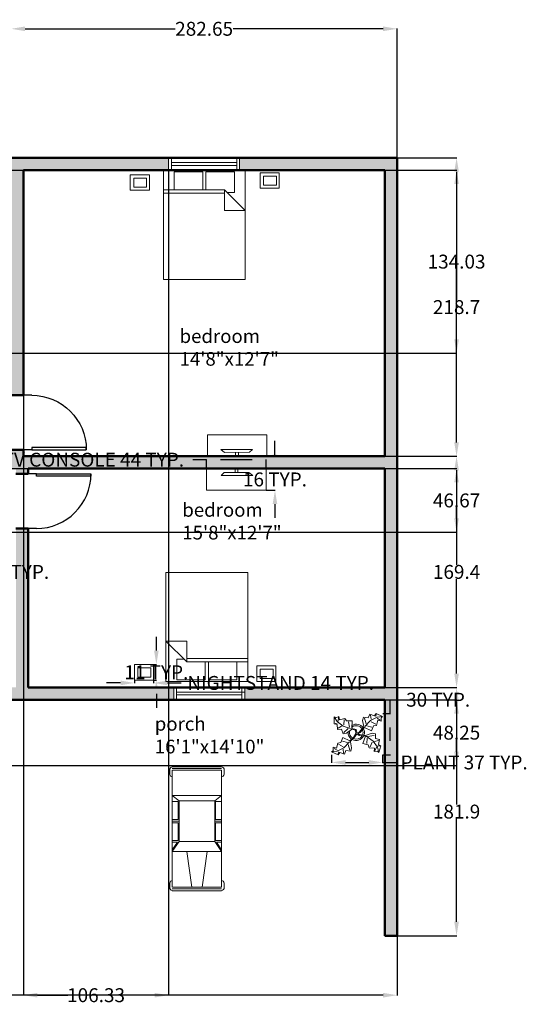
# Model space of a CAD drawing. Units: inches. Extents: x 12496 to 13538, y 6171 to 6892.
# Tile 6 of 6: x 13167 to 13538, y 6171 to 6892. Entities that reach past the tile are written whole.
import ezdxf

# ---------------------------------------------------------------- set-up
doc = ezdxf.new("R2010")
doc.units = ezdxf.units.IN
doc.header["$MEASUREMENT"] = 0
for name, color, linetype, lineweight in [('A-ANNO-DIMS', 2, 'Continuous', 18), ('A-AREA-IDEN', 7, 'Continuous', 25), ('A-DOOR', 3, 'Continuous', 25), ('A-EQPM-VEHI', 9, 'Continuous', 18), ('A-FURN', 8, 'Continuous', 18), ('A-GLAZ', 4, 'Continuous', 18), ('A-WALL', 7, 'Continuous', 50), ('L-PLNT', 3, 'Continuous', 18)]:
    doc.layers.add(name, color=color, linetype=linetype, lineweight=lineweight)
doc.layers.add('A-WALL-PATT', color=18, linetype='Continuous', lineweight=13, true_color=0x000000)
doc.styles.get("Standard").update_dxf_attribs({"font": 'arial.ttf'})
doc.dimstyles.get("Standard").update_dxf_attribs({"dimtxt": 10.18, "dimasz": 10.18, "dimexe": 0.18, "dimexo": 0.0625, "dimgap": 0.09, "dimtad": 0, "dimtih": 1, "dimtoh": 1, "dimdec": 0, "dimzin": 0, "dimdsep": 46, "dimlunit": 3, "dimtxsty": 'Standard', "dimcen": 0.09, "dimadec": 0, "dimazin": 0, "dimtfac": 1, "dimtdec": 0, "dimtofl": 0, "dimtmove": 0, "dimatfit": 3, "dimfxl": 1, "dimtolj": 1, "dimtzin": 0, "dimarcsym": 0})

# ---------------------------------------------------------------- blocks, each defined once
blk = doc.blocks.new('Bed - Queen')
for p, q in [((0, -80.00003), (0, 0)), ((0, 0), (59.99999, 0)), ((59.99999, 0), (59.99999, -80.00003)), ((7.99999, -1.2), (28.79998, -1.2)), ((7.99999, -14.4), (7.99999, -1.2)), ((28.79998, -1.2), (28.79998, -14.4)), ((31.19999, -1.2), (51.99999, -1.2)), ((31.19999, -14.4), (31.19999, -1.2)), ((51.99999, -1.2), (51.99999, -16.4)), ((0, -14.4), (44.8, -14.4)), ((59.99999, -29.6), (44.8, -14.4)), ((44.8, -14.4), (44.8, -29.6)), ((44.8, -16.8), (0, -16.8)), ((51.99999, -16.4), (46.79936, -16.4)), ((44.8, -29.6), (59.99999, -29.6)), ((59.99999, -80.00003), (0, -80.00003))]:
    blk.add_line(p, q)
blk = doc.blocks.new('Plant - Rubber or Philodendron')
for p, q in [((-16.2005, 11.4774), (-13.9899, 8.1064)), ((-16.2005, 11.4774), (-14.8639, 10.7964)), ((-16.0159, 6.3329), (-16.2005, 11.4774)), ((-14.8639, 10.7964), (-12.6195, 11.8975)), ((-13.9899, 8.1064), (-9.5434, 4.7185)), ((-13.3174, 8.325), (-13.0735, 11.0065)), ((-12.6195, 11.8975), (-12.1909, 9.4345)), ((-12.1909, 9.4345), (-8.3829, 10.3)), ((-8.8369, 9.409), (-9.0894, 5.6095)), ((-8.3829, 10.3), (-7.0549, 8.501)), ((-7.0549, 8.501), (-3.0284, 8.6941)), ((-4.8529, 4.012), (-5.7184, 7.82)), ((-3.0284, 8.6941), (-3.0709, 3.1041)), ((4.6914, 8.8812), (5.3859, 11.2828)), ((4.6914, 8.8812), (5.5014, 4.4831)), ((5.3859, 11.2828), (8.8871, 10.7908)), ((5.9878, 10.4842), (7.1971, 6.3869)), ((10.3916, 8.7942), (6.2847, 4.4028)), ((8.8871, 10.7908), (9.9809, 13.4933)), ((9.9809, 13.4933), (13.3837, 12.301)), ((15.3859, 11.3055), (10.3916, 8.7942)), ((10.5828, 12.6946), (10.8893, 9.7953)), ((14.2977, 6.1031), (10.9934, 7.9956)), ((13.3837, 12.301), (14.68, 13.9039)), ((14.5816, 13.2037), (14.3848, 11.8033)), ((14.68, 13.9039), (19.3848, 11.8146)), ((15.7909, 9.1065), (14.8995, 5.3044)), ((15.2875, 10.6053), (17.5907, 9.2105)), ((19.3848, 11.8146), (15.3859, 11.3055)), ((18.1925, 8.4119), (15.7909, 9.1065)), ((19.3848, 11.8146), (18.1868, 10.9119)), ((18.1868, 10.9119), (18.1925, 8.4119)), ((-14.0069, 5.8704), (-16.0159, 6.3329)), ((-15.3434, 6.5514), (-13.9984, 6.9884)), ((-13.5868, 2.2894), (-14.0069, 5.8704)), ((-10.6784, 2.491), (-13.5868, 2.2894)), ((-13.1329, 3.1804), (-10.6614, 4.727)), ((-9.5858, -0.8715), (-10.6784, 2.491)), ((-9.5434, 4.7185), (-4.1917, 2.9888)), ((-9.1318, 0.0195), (-5.9793, 2.9025)), ((-7.1228, -0.443), (-3.5248, 2.2131)), ((-3.5248, 2.2131), (-3.3011, 2.4355)), ((-3.3011, 2.4355), (-0.5306, 1.7947)), ((-3.0709, 3.1041), (0.0797, 2.3163)), ((-0.5306, 1.7947), (-0.2255, -0.5527)), ((-0.5306, 1.7947), (-0.5306, 1.7947)), ((0.0797, 2.3163), (0.4866, -0.031)), ((0.4866, -0.031), (2.1141, 0.2298)), ((2.1141, 0.2298), (5.4346, 3.9146)), ((6.1032, 3.6844), (2.8262, -0.031)), ((5.4346, 3.9146), (5.5014, 4.4831)), ((11.1089, 1.1958), (6.1032, 3.6844)), ((7.7005, 4.8881), (11.5025, 3.9967)), ((12.7005, 4.8994), (11.1089, 1.1958)), ((14.8995, 5.3044), (12.7005, 4.8994)), ((-11.3237, -7.2629), (-9.7321, -3.5593)), ((-6.3237, -7.2516), (-10.1257, -6.3602)), ((-9.7321, -3.5593), (-4.7264, -6.0479)), ((-7.1228, -0.443), (-9.5858, -0.8715)), ((-9.0148, -11.1577), (-4.9047, -6.8122)), ((-2.019, -3.6148), (-4.7264, -6.0479)), ((-4.1246, -6.8466), (-4.0579, -6.2781)), ((-3.3146, -11.2447), (-4.1246, -6.8466)), ((-4.0579, -6.2781), (-0.9375, -3.1608)), ((-2.019, -3.6148), (-0.2255, -0.5527)), ((-0.9375, -3.1608), (0.5883, -0.8135)), ((0.5883, -0.8135), (2.2447, -2.0916)), ((2.8262, -0.031), (1.3003, -0.5527)), ((1.3003, -0.5527), (2.4193, -1.4655)), ((2.2447, -2.0916), (6.7108, -2.6626)), ((2.4193, -1.4655), (6.895, -2.1175)), ((4.943, -7.9659), (6.7108, -2.6626)), ((11.6605, -0.5413), (6.895, -2.1175)), ((12.3677, -6.1981), (7.219, -2.6772)), ((8.125, -4.0768), (7.7715, -7.9659)), ((8.3544, -2.7453), (13.1973, -2.1704)), ((10.2463, -10.4408), (11.6605, -6.9053)), ((11.6605, -0.5413), (14.1354, -0.8948)), ((15.5496, -10.7943), (12.3677, -6.1981)), ((16.2567, -5.8446), (13.4283, -6.5517)), ((14.1354, -0.8948), (14.1354, -4.4304)), ((14.1354, -4.4304), (16.9638, -5.1375)), ((16.9638, -5.1375), (16.2567, -8.673)), ((-18.008, -14.1781), (-16.8101, -13.2754)), ((-18.008, -14.1781), (-14.0091, -13.669)), ((-13.3032, -16.2674), (-18.008, -14.1781)), ((-16.8157, -10.7754), (-14.4141, -11.4699)), ((-16.8101, -13.2754), (-16.8157, -10.7754)), ((-13.9107, -12.9688), (-16.2139, -11.574)), ((-14.4141, -11.4699), (-13.5228, -7.6679)), ((-14.0091, -13.669), (-9.0148, -11.1577)), ((-13.5228, -7.6679), (-11.3237, -7.2629)), ((-13.2048, -15.5672), (-13.008, -14.1668)), ((-12.921, -8.4665), (-9.6166, -10.359)), ((-9.206, -15.0581), (-9.5126, -12.1588)), ((-7.5103, -13.1543), (-8.6042, -15.8568)), ((-4.0092, -13.6463), (-7.5103, -13.1543)), ((-4.611, -12.8477), (-5.8203, -8.7504)), ((-3.3146, -11.2447), (-4.0092, -13.6463)), ((8.8321, -9.0266), (4.943, -7.9659)), ((9.5392, -11.1479), (8.8321, -9.0266)), ((13.4283, -11.5015), (9.5392, -11.1479)), ((13.0748, -13.9763), (13.4283, -11.5015)), ((15.5496, -13.6228), (13.0748, -13.9763)), ((14.8425, -10.7943), (13.7819, -13.2692)), ((16.6103, -14.6834), (15.5496, -10.7943)), ((16.6103, -14.6834), (15.5496, -13.6228)), ((17.3174, -9.7337), (15.9032, -9.7337)), ((16.2567, -8.673), (18.0245, -9.7337)), ((18.0245, -9.7337), (16.6103, -14.6834)), ((-12.0069, -14.6645), (-13.3032, -16.2674)), ((-8.6042, -15.8568), (-12.0069, -14.6645))]:
    blk.add_line(p, q)
for centre, radius, start, end in [((0.0308, 0.1664), 6, 178.6147, 235.1169), ((0.0308, 0.1664), 5, 168.1647, 238.6725), ((0, 0), 6.1275, 34.37569, 120.1028), ((-0.0601, -0.2075), 5.2461, 33.82192, 124.9414), ((-0.2664, 0.1682), 5.2775, 338.4094, 20.03007), ((-0.098, 0.1364), 6.1288, 341.2017, 26.09184), ((-0.0234, 0.3825), 6.1492, 242.5812, 331.2714), ((-0.1102, 0.4886), 5.2883, 247.3711, 327.472)]:
    blk.add_arc(centre, radius, start, end)
blk = doc.blocks.new('*U18')
for p, q in [((0.1, -0.4), (0.1, 38.3)), ((2.8, -0.4), (2.8, 38.3)), ((5.4, 42.3), (12.1, 42.3)), ((5.4, 38.3), (16.1, 38.3)), ((5.4, -0.4), (5.4, 38.2)), ((16.1, 38.3), (180.3, 38.3)), ((61.5, -0.4), (61.5, 38.3)), ((61.5, 38.3), (77.5, 27.6)), ((64.2, 38.3), (76.2, 30.3)), ((76.2, 30.3), (76.2, 38.3)), ((78.9, 38.3), (78.9, 29)), ((106.9, 29), (106.9, 38.3)), ((109.6, 27.6), (109.6, 38.3)), ((112.3, 38.3), (112.3, 29)), ((140.3, 29), (140.3, 38.3)), ((141.6, 27.6), (149.6, 38.3)), ((149.6, -0.4), (149.6, 38.3)), ((189.7, 38.3), (179, 38.3)), ((189.7, 42.3), (183, 42.3)), ((189.7, -0.4), (189.7, 38.2)), ((192.4, -0.4), (192.4, 38.3)), ((195, -0.4), (195, 38.3)), ((5.4, 7.6), (61.5, 15.6)), ((77.5, 27.6), (141.6, 27.6)), ((77.5, -0.4), (77.5, 27.6)), ((78.9, 29), (106.9, 29)), ((112.3, 29), (140.3, 29)), ((141.6, -0.4), (141.6, 27.6)), ((0.1, -0.4), (0.1, -39.2)), ((2.8, -0.4), (2.8, -39.1)), ((5.4, -0.4), (5.4, -39.1)), ((5.4, -8.4), (61.5, -16.4)), ((61.5, -0.4), (61.5, -39.1)), ((77.5, -0.4), (77.5, -28.5)), ((141.6, -0.4), (141.6, -28.5)), ((149.6, -0.4), (149.6, -39.1)), ((189.7, -0.4), (189.7, -39.1)), ((192.4, -0.4), (192.4, -39.1)), ((195, -0.4), (195, -39.2)), ((61.5, -39.1), (77.5, -28.5)), ((77.5, -28.5), (141.6, -28.5)), ((78.9, -39.1), (78.9, -29.8)), ((78.9, -29.8), (106.9, -29.8)), ((106.9, -29.8), (106.9, -39.1)), ((109.6, -28.5), (109.6, -39.1)), ((112.3, -29.8), (140.3, -29.8)), ((112.3, -39.1), (112.3, -29.8)), ((140.3, -29.8), (140.3, -39.1)), ((141.6, -28.5), (149.6, -39.1)), ((5.4, -39.1), (16.1, -39.1)), ((5.4, -43.1), (12.1, -43.1)), ((16.1, -39.1), (180.3, -39.1)), ((64.2, -39.1), (76.2, -31.1)), ((76.2, -31.1), (76.2, -39.1)), ((189.7, -39.1), (179, -39.1)), ((189.7, -43.1), (183, -43.1))]:
    blk.add_line(p, q)
for centre, radius, start, end in [((5.1, 37.3), 5.06, 85.6455, 168.0943), ((11.5, 37.6), 4.72, 8.1301, 81.87), ((183.7, 37.6), 4.72, 98.13, 171.8699), ((190.1, 37.3), 5.06, 11.9057, 94.3545), ((5.1, -38.1), 5.06, 191.9057, 274.3545), ((11.5, -38.5), 4.72, 278.13, 351.8699), ((183.7, -38.5), 4.72, 188.1301, 261.87), ((190.1, -38.1), 5.06, 265.6455, 348.0943)]:
    blk.add_arc(centre, radius, start, end)
blk = doc.blocks.new('*U2')
for p, q in [((0, 0), (0, -6)), ((40, 0), (40, -6))]:
    blk.add_line(p, q)
blk.add_lwpolyline([(0, 0), (0, 40), (1.75, 40), (1.75, 0)], close=True)
blk.add_arc((0, 0), 40, 0, 90)
blk = doc.blocks.new('TV-CONSOLE')
for p, q in [((10.88, 32.95), (10.88, 9.78)), ((10.88, 32.95), (12.91, 30.72)), ((12.91, 30.72), (13.04, 12.51)), ((12.98, 22.62), (15.84, 22.62)), ((12.98, 20.62), (15.84, 20.62)), ((10.88, 9.78), (13.04, 12.51))]:
    blk.add_line(p, q)
blk.add_lwpolyline([(15.84, 43.51), (0, 43.51), (0, 0), (15.84, 0)], close=True)
blk = doc.blocks.new('BEDSIDE-TABLE')
for points in [[(0, 11.4), (13.96, 11.4), (13.96, 0), (0, 0)], [(2.55, 8.94), (11.99, 8.94), (11.99, 2.21), (2.55, 2.21)]]:
    blk.add_lwpolyline(points, close=True)
blk = doc.blocks.new('WIN-48IN')
for p, q in [((0, 0), (0, 9)), ((2, 0), (2, 9)), ((50, 0), (50, 9)), ((52, 0), (52, 9)), ((2, 5.5), (50, 5.5)), ((2, 3.5), (50, 3.5))]:
    blk.add_line(p, q)
blk = doc.blocks.new('*D27')
at = {"layer": 'A-ANNO-DIMS', "color": 0, "lineweight": -2, "transparency": 16777216}
for p, q in [((13250.64, 6408.17), (13250.64, 6405.95)), ((13264.6, 6408.17), (13264.6, 6405.95)), ((13240.46, 6406.13), (13230.28, 6406.13)), ((13274.78, 6406.13), (13284.96, 6406.13))]:
    blk.add_line(p, q, dxfattribs=at)
at = {"layer": 'A-ANNO-DIMS', "color": 0, "transparency": 16777216}
for points in [[(13240.46, 6407.83), (13240.46, 6404.44), (13250.64, 6406.13)], [(13274.78, 6407.83), (13274.78, 6404.44), (13264.6, 6406.13)]]:
    blk.add_solid(points, dxfattribs=at)
at = {"layer": 'Defpoints', "color": 0, "transparency": 16777216}
for p in [(13250.64, 6408.23), (13264.6, 6408.23), (13264.6, 6406.13)]:
    blk.add_point(p, dxfattribs=at)
at = {"layer": 'A-ANNO-DIMS', "color": 0, "transparency": 16777216, "insert": (13357.78, 6406.13), "char_height": 10.18, "attachment_point": 5}
blk.add_mtext('\\A1;NIGHTSTAND 14 TYP.', dxfattribs=at)
blk = doc.blocks.new('*D28')
at = {"layer": 'A-ANNO-DIMS', "color": 0, "lineweight": -2, "transparency": 16777216}
for p, q in [((13266.7, 6429.81), (13266.7, 6439.99)), ((13264.67, 6419.63), (13266.88, 6419.63)), ((13264.67, 6408.23), (13266.88, 6408.23)), ((13266.7, 6398.05), (13266.7, 6387.87))]:
    blk.add_line(p, q, dxfattribs=at)
at = {"layer": 'A-ANNO-DIMS', "color": 0, "transparency": 16777216}
for points in [[(13265, 6429.81), (13268.4, 6429.81), (13266.7, 6419.63)], [(13265, 6398.05), (13268.4, 6398.05), (13266.7, 6408.23)]]:
    blk.add_solid(points, dxfattribs=at)
at = {"layer": 'Defpoints', "color": 0, "transparency": 16777216}
for p in [(13264.6, 6419.63), (13266.7, 6419.63), (13264.6, 6408.23)]:
    blk.add_point(p, dxfattribs=at)
at = {"layer": 'A-ANNO-DIMS', "color": 0, "transparency": 16777216, "insert": (13266.7, 6413.93), "char_height": 10.18, "attachment_point": 5}
blk.add_mtext('\\A1;11 TYP.', dxfattribs=at)
blk = doc.blocks.new('*D29')
at = {"layer": 'A-ANNO-DIMS', "color": 0, "lineweight": -2, "transparency": 16777216}
for p, q in [((13303.55, 6569.73), (13293.37, 6569.73)), ((13303.55, 6563.27), (13303.55, 6569.91)), ((13336.87, 6569.73), (13313.73, 6569.73)), ((13347.05, 6563.27), (13347.05, 6569.91))]:
    blk.add_line(p, q, dxfattribs=at)
at = {"layer": 'A-ANNO-DIMS', "color": 0, "transparency": 16777216}
for points in [[(13313.73, 6571.43), (13313.73, 6568.03), (13303.55, 6569.73)], [(13336.87, 6571.43), (13336.87, 6568.03), (13347.05, 6569.73)]]:
    blk.add_solid(points, dxfattribs=at)
at = {"layer": 'Defpoints', "color": 0, "transparency": 16777216}
for p in [(13303.55, 6569.73), (13303.55, 6563.2), (13347.05, 6563.2)]:
    blk.add_point(p, dxfattribs=at)
at = {"layer": 'A-ANNO-DIMS', "color": 0, "transparency": 16777216, "insert": (13220.56, 6569.73), "char_height": 10.18, "attachment_point": 5}
blk.add_mtext('\\A1;TV CONSOLE 44 TYP.', dxfattribs=at)
blk = doc.blocks.new('*D30')
at = {"layer": 'A-ANNO-DIMS', "color": 0, "lineweight": -2, "transparency": 16777216}
for p, q in [((13353.58, 6573.38), (13353.58, 6583.56)), ((13347.12, 6563.2), (13353.76, 6563.2)), ((13347.12, 6547.36), (13353.76, 6547.36)), ((13353.58, 6537.18), (13353.58, 6527))]:
    blk.add_line(p, q, dxfattribs=at)
at = {"layer": 'A-ANNO-DIMS', "color": 0, "transparency": 16777216}
for points in [[(13351.88, 6573.38), (13355.28, 6573.38), (13353.58, 6563.2)], [(13351.88, 6537.18), (13355.28, 6537.18), (13353.58, 6547.36)]]:
    blk.add_solid(points, dxfattribs=at)
at = {"layer": 'Defpoints', "color": 0, "transparency": 16777216}
for p in [(13347.05, 6563.2), (13353.58, 6563.2), (13347.05, 6547.36)]:
    blk.add_point(p, dxfattribs=at)
at = {"layer": 'A-ANNO-DIMS', "color": 0, "transparency": 16777216, "insert": (13353.58, 6555.28), "char_height": 10.18, "attachment_point": 5}
blk.add_mtext('\\A1;16 TYP.', dxfattribs=at)
blk = doc.blocks.new('*D35')
at = {"layer": 'A-ANNO-DIMS', "color": 0, "lineweight": -2, "transparency": 16777216}
for p, q in [((13395.08, 6353.41), (13395.08, 6347.68)), ((13432.47, 6353.41), (13432.47, 6347.68)), ((13405.26, 6347.86), (13422.29, 6347.86)), ((13432.47, 6347.86), (13442.65, 6347.86))]:
    blk.add_line(p, q, dxfattribs=at)
at = {"layer": 'A-ANNO-DIMS', "color": 0, "transparency": 16777216}
for points in [[(13405.26, 6349.56), (13405.26, 6346.17), (13395.08, 6347.86)], [(13422.29, 6349.56), (13422.29, 6346.17), (13432.47, 6347.86)]]:
    blk.add_solid(points, dxfattribs=at)
at = {"layer": 'Defpoints', "color": 0, "transparency": 16777216}
for p in [(13395.08, 6353.47), (13432.47, 6353.47), (13432.47, 6347.86)]:
    blk.add_point(p, dxfattribs=at)
at = {"layer": 'A-ANNO-DIMS', "color": 0, "transparency": 16777216, "insert": (13492.16, 6347.86), "char_height": 10.18, "attachment_point": 5}
blk.add_mtext('\\A1;PLANT 37 TYP.', dxfattribs=at)
blk = doc.blocks.new('*D36')
at = {"layer": 'A-ANNO-DIMS', "color": 0, "lineweight": -2, "transparency": 16777216}
for p, q in [((13438.08, 6383.64), (13438.08, 6393.82)), ((13438.08, 6393.82), (13448.26, 6393.82)), ((13432.53, 6383.64), (13438.26, 6383.64)), ((13438.08, 6363.65), (13438.08, 6373.46)), ((13432.53, 6353.47), (13438.26, 6353.47))]:
    blk.add_line(p, q, dxfattribs=at)
at = {"layer": 'A-ANNO-DIMS', "color": 0, "transparency": 16777216}
for points in [[(13436.38, 6373.46), (13439.77, 6373.46), (13438.08, 6383.64)], [(13436.38, 6363.65), (13439.77, 6363.65), (13438.08, 6353.47)]]:
    blk.add_solid(points, dxfattribs=at)
at = {"layer": 'Defpoints', "color": 0, "transparency": 16777216}
for p in [(13432.47, 6383.64), (13438.08, 6383.64), (13432.47, 6353.47)]:
    blk.add_point(p, dxfattribs=at)
at = {"layer": 'A-ANNO-DIMS', "color": 0, "transparency": 16777216, "insert": (13473.12, 6393.82), "char_height": 10.18, "attachment_point": 5}
blk.add_mtext('\\A1;30 TYP.', dxfattribs=at)
blk = doc.blocks.new('*D43')
at = {"layer": 'A-ANNO-DIMS', "color": 0, "lineweight": -2, "transparency": 16777216}
for p, q in [((13005.46, 6500.01), (13005.46, 6487.3)), ((13089.46, 6500.01), (13089.46, 6487.3)), ((13015.64, 6487.48), (13079.28, 6487.48)), ((13089.46, 6487.48), (13099.64, 6487.48))]:
    blk.add_line(p, q, dxfattribs=at)
at = {"layer": 'A-ANNO-DIMS', "color": 0, "transparency": 16777216}
for points in [[(13015.64, 6489.17), (13015.64, 6485.78), (13005.46, 6487.48)], [(13079.28, 6489.17), (13079.28, 6485.78), (13089.46, 6487.48)]]:
    blk.add_solid(points, dxfattribs=at)
at = {"layer": 'Defpoints', "color": 0, "transparency": 16777216}
for p in [(13005.46, 6500.08), (13089.46, 6500.08), (13089.46, 6487.48)]:
    blk.add_point(p, dxfattribs=at)
at = {"layer": 'A-ANNO-DIMS', "color": 0, "transparency": 16777216, "insert": (13145.82, 6487.48), "char_height": 10.18, "attachment_point": 5}
blk.add_mtext('\\A1;SOFA 84 TYP.', dxfattribs=at)
blk = doc.blocks.new('*D59')
at = {"layer": 'A-ANNO-DIMS', "color": 0, "lineweight": -2, "transparency": 16777216}
for p, q in [((12622.17, 6220.83), (12622.17, 6177.12)), ((13443.03, 6220.83), (13443.03, 6177.12)), ((12632.35, 6177.3), (13015.32, 6177.3)), ((13432.85, 6177.3), (13049.88, 6177.3))]:
    blk.add_line(p, q, dxfattribs=at)
at = {"layer": 'A-ANNO-DIMS', "color": 0, "transparency": 16777216}
for points in [[(12632.35, 6179), (12632.35, 6175.6), (12622.17, 6177.3)], [(13432.85, 6179), (13432.85, 6175.6), (13443.03, 6177.3)]]:
    blk.add_solid(points, dxfattribs=at)
at = {"layer": 'Defpoints', "color": 0, "transparency": 16777216}
for p in [(12622.17, 6220.89), (13443.03, 6220.89), (13443.03, 6177.3)]:
    blk.add_point(p, dxfattribs=at)
at = {"layer": 'A-ANNO-DIMS', "color": 0, "transparency": 16777216, "insert": (13032.6, 6177.3), "char_height": 10.18, "attachment_point": 5}
blk.add_mtext('\\A1;820.9', dxfattribs=at)
blk = doc.blocks.new('*D64')
at = {"layer": 'A-ANNO-DIMS', "color": 0, "lineweight": -2, "transparency": 16777216}
for p, q in [((13160.38, 6781.96), (13160.38, 6885.67)), ((13170.56, 6885.49), (13280.36, 6885.49)), ((13432.85, 6885.49), (13323.05, 6885.49)), ((13443.03, 6790.96), (13443.03, 6885.67))]:
    blk.add_line(p, q, dxfattribs=at)
at = {"layer": 'A-ANNO-DIMS', "color": 0, "transparency": 16777216}
for points in [[(13170.56, 6887.18), (13170.56, 6883.79), (13160.38, 6885.49)], [(13432.85, 6887.18), (13432.85, 6883.79), (13443.03, 6885.49)]]:
    blk.add_solid(points, dxfattribs=at)
at = {"layer": 'Defpoints', "color": 0, "transparency": 16777216}
for p in [(13443.03, 6885.49), (13443.03, 6790.89), (13160.38, 6781.89)]:
    blk.add_point(p, dxfattribs=at)
at = {"layer": 'A-ANNO-DIMS', "color": 0, "transparency": 16777216, "insert": (13301.7, 6885.49), "char_height": 10.18, "attachment_point": 5}
blk.add_mtext('\\A1;282.65', dxfattribs=at)
blk = doc.blocks.new('*D67')
at = {"layer": 'A-ANNO-DIMS', "color": 0, "lineweight": -2, "transparency": 16777216}
for p, q in [((13443.09, 6790.89), (13486.8, 6790.89)), ((13486.62, 6780.71), (13486.62, 6686.84)), ((13486.62, 6582.38), (13486.62, 6676.26)), ((13434.09, 6572.2), (13486.8, 6572.2))]:
    blk.add_line(p, q, dxfattribs=at)
at = {"layer": 'A-ANNO-DIMS', "color": 0, "transparency": 16777216}
for points in [[(13484.92, 6780.71), (13488.32, 6780.71), (13486.62, 6790.89)], [(13484.92, 6582.38), (13488.32, 6582.38), (13486.62, 6572.2)]]:
    blk.add_solid(points, dxfattribs=at)
at = {"layer": 'Defpoints', "color": 0, "transparency": 16777216}
for p in [(13443.03, 6790.89), (13434.03, 6572.2), (13486.62, 6572.2)]:
    blk.add_point(p, dxfattribs=at)
at = {"layer": 'A-ANNO-DIMS', "color": 0, "transparency": 16777216, "insert": (13486.62, 6681.55), "char_height": 10.18, "attachment_point": 5}
blk.add_mtext('\\A1;218.7', dxfattribs=at)
blk = doc.blocks.new('*D68')
at = {"layer": 'A-ANNO-DIMS', "color": 0, "lineweight": -2, "transparency": 16777216}
for p, q in [((13434.09, 6572.2), (13486.8, 6572.2)), ((13486.62, 6562.02), (13486.62, 6492.79)), ((13486.62, 6412.97), (13486.62, 6482.21)), ((13434.09, 6402.79), (13486.8, 6402.79))]:
    blk.add_line(p, q, dxfattribs=at)
at = {"layer": 'A-ANNO-DIMS', "color": 0, "transparency": 16777216}
for points in [[(13484.92, 6562.02), (13488.32, 6562.02), (13486.62, 6572.2)], [(13484.92, 6412.97), (13488.32, 6412.97), (13486.62, 6402.79)]]:
    blk.add_solid(points, dxfattribs=at)
at = {"layer": 'Defpoints', "color": 0, "transparency": 16777216}
for p in [(13434.03, 6572.2), (13434.03, 6402.79), (13486.62, 6402.79)]:
    blk.add_point(p, dxfattribs=at)
at = {"layer": 'A-ANNO-DIMS', "color": 0, "transparency": 16777216, "insert": (13486.62, 6487.5), "char_height": 10.18, "attachment_point": 5}
blk.add_mtext('\\A1;169.4', dxfattribs=at)
blk = doc.blocks.new('*D69')
at = {"layer": 'A-ANNO-DIMS', "color": 0, "lineweight": -2, "transparency": 16777216}
for p, q in [((13434.09, 6402.79), (13486.8, 6402.79)), ((13486.62, 6392.61), (13486.62, 6317.13)), ((13486.62, 6231.07), (13486.62, 6306.56)), ((13443.09, 6220.89), (13486.8, 6220.89))]:
    blk.add_line(p, q, dxfattribs=at)
at = {"layer": 'A-ANNO-DIMS', "color": 0, "transparency": 16777216}
for points in [[(13484.92, 6392.61), (13488.32, 6392.61), (13486.62, 6402.79)], [(13484.92, 6231.07), (13488.32, 6231.07), (13486.62, 6220.89)]]:
    blk.add_solid(points, dxfattribs=at)
at = {"layer": 'Defpoints', "color": 0, "transparency": 16777216}
for p in [(13434.03, 6402.79), (13443.03, 6220.89), (13486.62, 6220.89)]:
    blk.add_point(p, dxfattribs=at)
at = {"layer": 'A-ANNO-DIMS', "color": 0, "transparency": 16777216, "insert": (13486.62, 6311.84), "char_height": 10.18, "attachment_point": 5}
blk.add_mtext('\\A1;181.9', dxfattribs=at)
blk = doc.blocks.new('*D70')
at = {"layer": 'A-ANNO-DIMS', "color": 0, "lineweight": -2, "transparency": 16777216}
for p, q in [((12880.13, 6781.89), (13486.8, 6781.89)), ((13486.62, 6771.71), (13486.62, 6720.17)), ((13486.62, 6658.04), (13486.62, 6709.59)), ((12880.13, 6647.86), (13486.8, 6647.86))]:
    blk.add_line(p, q, dxfattribs=at)
at = {"layer": 'A-ANNO-DIMS', "color": 0, "transparency": 16777216}
for points in [[(13484.92, 6771.71), (13488.32, 6771.71), (13486.62, 6781.89)], [(13484.92, 6658.04), (13488.32, 6658.04), (13486.62, 6647.86)]]:
    blk.add_solid(points, dxfattribs=at)
at = {"layer": 'Defpoints', "color": 0, "transparency": 16777216}
for p in [(12880.07, 6781.89), (12880.07, 6647.86), (13486.62, 6647.86)]:
    blk.add_point(p, dxfattribs=at)
at = {"layer": 'A-ANNO-DIMS', "color": 0, "transparency": 16777216, "insert": (13486.62, 6714.88), "char_height": 10.18, "attachment_point": 5}
blk.add_mtext('\\A1;134.03', dxfattribs=at)
blk = doc.blocks.new('*D72')
at = {"layer": 'A-ANNO-DIMS', "color": 0, "lineweight": -2, "transparency": 16777216}
for p, q in [((12734.45, 6393.81), (13486.8, 6393.81)), ((13486.62, 6383.63), (13486.62, 6374.97)), ((13486.62, 6355.74), (13486.62, 6364.4)), ((12734.45, 6345.56), (13486.8, 6345.56))]:
    blk.add_line(p, q, dxfattribs=at)
at = {"layer": 'A-ANNO-DIMS', "color": 0, "transparency": 16777216}
for points in [[(13484.92, 6383.63), (13488.32, 6383.63), (13486.62, 6393.81)], [(13484.92, 6355.74), (13488.32, 6355.74), (13486.62, 6345.56)]]:
    blk.add_solid(points, dxfattribs=at)
at = {"layer": 'Defpoints', "color": 0, "transparency": 16777216}
for p in [(12734.39, 6393.81), (13486.62, 6393.81), (12734.39, 6345.56)]:
    blk.add_point(p, dxfattribs=at)
at = {"layer": 'A-ANNO-DIMS', "color": 0, "transparency": 16777216, "insert": (13486.62, 6369.69), "char_height": 10.18, "attachment_point": 5}
blk.add_mtext('\\A1;48.25', dxfattribs=at)
blk = doc.blocks.new('*D76')
at = {"layer": 'A-ANNO-DIMS', "color": 0, "lineweight": -2, "transparency": 16777216}
for p, q in [((12721.51, 6563.2), (13486.8, 6563.2)), ((13486.62, 6553.02), (13486.62, 6545.16)), ((13486.62, 6526.72), (13486.62, 6534.58)), ((12721.51, 6516.54), (13486.8, 6516.54))]:
    blk.add_line(p, q, dxfattribs=at)
at = {"layer": 'A-ANNO-DIMS', "color": 0, "transparency": 16777216}
for points in [[(13484.92, 6553.02), (13488.32, 6553.02), (13486.62, 6563.2)], [(13484.92, 6526.72), (13488.32, 6526.72), (13486.62, 6516.54)]]:
    blk.add_solid(points, dxfattribs=at)
at = {"layer": 'Defpoints', "color": 0, "transparency": 16777216}
for p in [(12721.45, 6563.2), (13486.62, 6563.2), (12721.45, 6516.54)]:
    blk.add_point(p, dxfattribs=at)
at = {"layer": 'A-ANNO-DIMS', "color": 0, "transparency": 16777216, "insert": (13486.62, 6539.87), "char_height": 10.18, "attachment_point": 5}
blk.add_mtext('\\A1;46.67', dxfattribs=at)
blk = doc.blocks.new('*D83')
at = {"layer": 'A-ANNO-DIMS', "color": 0, "lineweight": -2, "transparency": 16777216}
for p, q in [((13169.38, 6781.83), (13169.38, 6177.12)), ((13275.7, 6781.83), (13275.7, 6177.12)), ((13179.56, 6177.3), (13201.8, 6177.3)), ((13265.52, 6177.3), (13243.28, 6177.3))]:
    blk.add_line(p, q, dxfattribs=at)
at = {"layer": 'A-ANNO-DIMS', "color": 0, "transparency": 16777216}
for points in [[(13179.56, 6179), (13179.56, 6175.6), (13169.38, 6177.3)], [(13265.52, 6179), (13265.52, 6175.6), (13275.7, 6177.3)]]:
    blk.add_solid(points, dxfattribs=at)
at = {"layer": 'Defpoints', "color": 0, "transparency": 16777216}
for p in [(13169.38, 6781.89), (13275.7, 6781.89), (13275.7, 6177.3)]:
    blk.add_point(p, dxfattribs=at)
at = {"layer": 'A-ANNO-DIMS', "color": 0, "transparency": 16777216, "insert": (13222.54, 6177.3), "char_height": 10.18, "attachment_point": 5}
blk.add_mtext('\\A1;106.33', dxfattribs=at)

msp = doc.modelspace()

# ---------------------------------------------------------------- hatches: boundary and pattern name
at = {"layer": 'A-WALL-PATT'}
h = msp.add_hatch(color=256, dxfattribs=at)
h.dxf.hatch_style = 1
h.paths.add_polyline_path([(12631.1731, 6781.8943), (12725.1219, 6781.8943), (12725.1219, 6790.8943), (12622.1731, 6790.8943), (12622.1731, 6551.6486), (12631.1731, 6551.6486), (12631.1731, 6563.2028), (12825.2657, 6563.2028), (12825.2657, 6572.2028), (12631.1731, 6572.2028)])
h.paths.add_polyline_path([(12941.4956, 6790.8943), (12777.1219, 6790.8943), (12777.1219, 6781.8943), (12871.0706, 6781.8943), (12871.0706, 6616.9323), (12880.0706, 6616.9323), (12880.0706, 6638.8628), (12890.9211, 6638.8628), (12890.9211, 6647.8628), (12880.0706, 6647.8628), (12880.0706, 6781.8943), (12941.4956, 6781.8943)])
h.paths.add_polyline_path([(13039.9206, 6781.8943), (13086.1485, 6781.8943), (13086.1485, 6790.8943), (12969.4956, 6790.8943), (12969.4956, 6781.8943), (13030.9206, 6781.8943), (13030.9206, 6647.8628), (13039.9206, 6647.8628)])
h.paths.add_polyline_path([(13275.7025, 6790.8943), (13114.1485, 6790.8943), (13114.1485, 6781.8943), (13160.3765, 6781.8943), (13160.3765, 6647.8628), (13088.7069, 6647.8628), (13088.7069, 6638.8628), (13160.3765, 6638.8628), (13160.3765, 6616.9323), (13169.3765, 6616.9323), (13169.3765, 6781.8943), (13275.7025, 6781.8943)])
h = msp.add_hatch(color=256, dxfattribs=at)
h.dxf.hatch_style = 1
h.paths.add_polyline_path([(13443.0285, 6790.8943), (13327.7025, 6790.8943), (13327.7025, 6781.8943), (13434.0285, 6781.8943), (13434.0285, 6572.2028), (13169.3765, 6572.2028), (13169.3765, 6576.9323), (13160.3765, 6576.9323), (13160.3765, 6563.2028), (13163.811, 6563.2028), (13163.811, 6559.305), (13172.811, 6559.305), (13172.811, 6563.2028), (13434.0285, 6563.2028), (13434.0285, 6402.794), (13331.4198, 6402.794), (13331.4198, 6393.8103), (13434.0285, 6393.8103), (13434.0285, 6220.8943), (13443.0285, 6220.8943)])
h.paths.add_polyline_path([(13172.811, 6519.305), (13163.811, 6519.305), (13163.811, 6402.8103), (12944.6655, 6402.8103), (12944.6655, 6393.8103), (13100.0985, 6393.8103), (13100.0985, 6312.5223), (13035.7682, 6312.5223), (13035.7682, 6303.5223), (13109.0985, 6303.5223), (13109.0985, 6393.8103), (13279.4198, 6393.8103), (13279.4198, 6402.8103), (13172.811, 6402.8103)])
h.paths.add_polyline_path([(13109.0985, 6229.8943), (12846.603, 6229.8943), (12846.603, 6303.5223), (12853.6371, 6303.5223), (12853.6371, 6312.5223), (12846.603, 6312.5223), (12846.603, 6393.8103), (12872.7237, 6393.8103), (12872.7237, 6402.8103), (12846.603, 6402.8103), (12837.603, 6402.8103), (12837.603, 6229.8943), (12760.3881, 6229.8943), (12760.3881, 6220.8943), (13109.0985, 6220.8943)])
h.paths.add_polyline_path([(12708.3881, 6229.8943), (12631.1731, 6229.8943), (12631.1731, 6336.5598), (12702.8967, 6336.5598), (12702.8967, 6345.5598), (12631.1731, 6345.5598), (12631.1731, 6355.6851), (12622.1731, 6355.6851), (12622.1731, 6220.8943), (12708.3881, 6220.8943)])
h.paths.add_polyline_path([(12743.3881, 6402.8103), (12631.1731, 6402.8103), (12631.1731, 6523.6486), (12622.1731, 6523.6486), (12622.1731, 6383.6851), (12631.1731, 6383.6851), (12631.1731, 6393.8103), (12734.3881, 6393.8103), (12734.3881, 6345.5598), (12731.8151, 6345.5598), (12731.8151, 6336.5598), (12734.3881, 6336.5598), (12743.3881, 6336.5598)])
h.paths.add_polyline_path([(13039.9206, 6572.2028), (13039.9206, 6638.8628), (13048.7069, 6638.8628), (13048.7069, 6647.8628), (13039.9206, 6647.8628), (12930.9211, 6647.8628), (12930.9211, 6638.8628), (13030.9206, 6638.8628), (13030.9206, 6572.2028), (12880.0706, 6572.2028), (12880.0706, 6576.9323), (12871.0706, 6576.9323), (12871.0706, 6572.2028), (12865.2657, 6572.2028), (12865.2657, 6563.2028), (13039.9206, 6563.2028)])
h.paths.add_polyline_path([(13039.9206, 6781.8943), (13086.1485, 6781.8943), (13086.1485, 6790.8943), (12969.4956, 6790.8943), (12969.4956, 6781.8943), (13030.9206, 6781.8943), (13030.9206, 6647.8628), (13039.9206, 6647.8628)])
h.paths.add_polyline_path([(13169.3765, 6781.8943), (13275.7025, 6781.8943), (13275.7025, 6790.8943), (13114.1485, 6790.8943), (13114.1485, 6781.8943), (13160.3765, 6781.8943), (13160.3765, 6647.8628), (13088.7069, 6647.8628), (13088.7069, 6638.8628), (13160.3765, 6638.8628), (13160.3765, 6616.9323), (13169.3765, 6616.9323)])

# ---------------------------------------------------------------- linework, layer by layer
at = {"layer": 'A-GLAZ'}
for p, q in [((13279.4198, 6402.794), (13279.4198, 6394.1344)), ((13281.4198, 6402.794), (13281.4198, 6394.1344)), ((13329.4198, 6402.794), (13329.4198, 6394.1344)), ((13331.4198, 6402.794), (13331.4198, 6394.1344)), ((13281.4198, 6399.4642), (13331.4198, 6399.4642)), ((13281.4198, 6397.4642), (13329.4198, 6397.4642))]:
    msp.add_line(p, q, dxfattribs=at)
at = {"layer": 'A-WALL'}
for p, q in [((12622.1731, 6790.8943), (13443.0285, 6790.8943)), ((13443.0285, 6790.8943), (13443.0285, 6220.8943)), ((13169.3765, 6781.8943), (13434.0285, 6781.8943)), ((13169.3765, 6616.9323), (13169.3765, 6781.8943)), ((13434.0285, 6781.8943), (13434.0285, 6572.2028)), ((13169.3765, 6616.9323), (13160.3765, 6616.9323)), ((13169.3765, 6576.9323), (13160.3765, 6576.9323)), ((13169.3765, 6572.2028), (13169.3765, 6576.9323)), ((13169.3765, 6572.2028), (13434.0285, 6572.2028)), ((13172.811, 6559.305), (13163.811, 6559.305)), ((13172.811, 6563.2028), (13172.811, 6559.305)), ((13172.811, 6563.2028), (13434.0285, 6563.2028)), ((13434.0285, 6563.2028), (13434.0285, 6402.794)), ((13172.811, 6519.305), (13163.811, 6519.305)), ((13172.811, 6519.305), (13172.811, 6402.8103)), ((13172.811, 6402.8103), (13329.4198, 6402.8103)), ((13329.4198, 6402.794), (13434.0285, 6402.794)), ((13109.0985, 6393.8103), (13434.0285, 6393.8103)), ((13434.0285, 6393.8103), (13434.0285, 6220.8943)), ((13434.0285, 6220.8943), (13443.0285, 6220.8943))]:
    msp.add_line(p, q, dxfattribs=at)

# ---------------------------------------------------------------- block references
at = {"layer": 'A-DOOR', "xscale": -1, "rotation": 270}
msp.add_blockref('*U2', (13175.3765, 6576.9323), dxfattribs=at)
at = {"layer": 'A-DOOR', "rotation": 270}
msp.add_blockref('*U2', (13178.811, 6559.305), dxfattribs=at)
at = {"layer": 'A-EQPM-VEHI', "xscale": 0.4659763824496534, "yscale": 0.4659763824496534, "zscale": 0.4659763824496534, "rotation": 90}
msp.add_blockref('*U18', (13296.2411, 6253.8336), dxfattribs=at)
at = {"layer": 'A-FURN'}
for name, p in [('BEDSIDE-TABLE', (13247.602, 6767.19)), ('Bed - Queen', (13271.8602, 6781.8943)), ('BEDSIDE-TABLE', (13342.6909, 6768.6234)), ('BEDSIDE-TABLE', (13250.6412, 6408.2292)), ('BEDSIDE-TABLE', (13340.3073, 6407.2277))]:
    msp.add_blockref(name, p, dxfattribs=at)
for name, p, rotation in [('TV-CONSOLE', (13304.1643, 6588.0438), 269.9999999999911), ('TV-CONSOLE', (13347.0541, 6547.3618), 89.99999999998747), ('Bed - Queen', (13333.7122, 6407.1237), 180)]:
    msp.add_blockref(name, p, dxfattribs=dict(at, rotation=rotation))
at = {"layer": 'A-GLAZ', "rotation": 180}
msp.add_blockref('WIN-48IN', (13327.7024, 6790.8947), dxfattribs=at)
at = {"layer": 'L-PLNT'}
msp.add_blockref('Plant - Rubber or Philodendron', (13413.0841, 6369.7398), dxfattribs=at)

# ---------------------------------------------------------------- texts
at = {"layer": 'A-AREA-IDEN', "char_height": 10, "attachment_point": 1}
for s, insert in [('bedroom\\P14\'8"x12\'7"', (13283.721, 6665.2679)), ('bedroom\\P15\'8"x12\'7"', (13285.7209, 6537.9358)), ('porch\\P16\'1"x14\'10"', (13265.5382, 6381.1634))]:
    msp.add_mtext_dynamic_manual_height_columns(s, width=261.947845, gutter_width=1, heights=[0], dxfattribs=dict(at, insert=insert))

# ---------------------------------------------------------------- dimensions: what is measured, and where the dimension line sits
at = {"layer": 'A-ANNO-DIMS'}
for base, p1, p2, override, picture, middle in [((13443.0285, 6885.4873), (13160.3765, 6781.8943), (13443.0285, 6790.8943), {"dimdec": 2, "dimlfac": 1, "dimrnd": 0, "dimzin": 0, "dimdsep": 46, "dimlunit": 2}, '*D64', (13301.7025, 6885.4873)), ((13275.7025, 6177.3013), (13169.3765, 6781.8943), (13275.7025, 6781.8943), {"dimdec": 2, "dimlfac": 1, "dimrnd": 0, "dimzin": 0, "dimdsep": 46, "dimlunit": 2}, '*D83', (13222.5395, 6177.3013)), ((13443.0285, 6177.3013), (12622.1731, 6220.8943), (13443.0285, 6220.8943), {"dimdec": 1, "dimlfac": 1, "dimrnd": 0, "dimzin": 0, "dimdsep": 46, "dimlunit": 2}, '*D59', (13032.6008, 6177.3013))]:
    dim = msp.add_linear_dim(base=base, p1=p1, p2=p2, dimstyle='Standard', override=override, dxfattribs=at)
    dim.commit()
    dim.dimension.update_dxf_attribs({"geometry": picture, "text_midpoint": middle})
for base, p1, p2, override, picture, middle in [((13486.6215, 6572.2028), (13443.0285, 6790.8943), (13434.0285, 6572.2028), {"dimdec": 1, "dimlfac": 1, "dimrnd": 0, "dimzin": 0, "dimdsep": 46, "dimlunit": 2}, '*D67', (13486.6215, 6681.5486)), ((13486.6215, 6647.8628), (12880.0706, 6781.8943), (12880.0706, 6647.8628), {"dimdec": 2, "dimlfac": 1, "dimrnd": 0, "dimzin": 0, "dimdsep": 46, "dimlunit": 2}, '*D70', (13486.6215, 6714.8786)), ((13486.6215, 6402.794), (13434.0285, 6572.2028), (13434.0285, 6402.794), {"dimdec": 1, "dimlfac": 1, "dimrnd": 0, "dimzin": 0, "dimdsep": 46, "dimlunit": 2}, '*D68', (13486.6215, 6487.4984)), ((13486.6215, 6563.2028), (12721.4504, 6516.5354), (12721.4504, 6563.2028), {"dimdec": 2, "dimlfac": 1, "dimrnd": 0, "dimzin": 0, "dimdsep": 46, "dimlunit": 2}, '*D76', (13486.6215, 6539.8691)), ((13486.6215, 6220.8943), (13434.0285, 6402.794), (13443.0285, 6220.8943), {"dimdec": 1, "dimlfac": 1, "dimrnd": 0, "dimzin": 0, "dimdsep": 46, "dimlunit": 2}, '*D69', (13486.6215, 6311.8442)), ((13486.6215, 6393.8103), (12734.3881, 6345.5598), (12734.3881, 6393.8103), {"dimdec": 2, "dimlfac": 1, "dimrnd": 0, "dimzin": 0, "dimdsep": 46, "dimlunit": 2}, '*D72', (13486.6215, 6369.6851))]:
    dim = msp.add_linear_dim(base=base, p1=p1, p2=p2, angle=90, dimstyle='Standard', override=override, dxfattribs=at)
    dim.commit()
    dim.dimension.update_dxf_attribs({"geometry": picture, "text_midpoint": middle})
for base, p1, p2, angle, text, picture, middle in [((13303.5465, 6569.729), (13347.0546, 6563.2028), (13303.5465, 6563.2028), 180, 'TV CONSOLE <> TYP.', '*D29', (13220.5618, 6569.729)), ((13353.5808, 6563.2028), (13347.0546, 6547.3621), (13347.0546, 6563.2028), 90, '<> TYP.', '*D30', (13353.5808, 6555.2824)), ((13266.6991, 6419.6318), (13264.6046, 6408.229), (13264.6046, 6419.6318), 90, '<> TYP.', '*D28', (13266.6991, 6413.9304)), ((13438.0779, 6383.6437), (13432.4689, 6353.4724), (13432.4689, 6383.6437), 90, '<> TYP.', '*D36', (13473.1208, 6393.8237))]:
    dim = msp.add_linear_dim(base=base, p1=p1, p2=p2, angle=angle, text=text, dimstyle='Standard', override={"dimdec": 0, "dimlfac": 1, "dimrnd": 0, "dimzin": 0, "dimdsep": 46, "dimlunit": 2}, dxfattribs=at)
    dim.commit()
    dim.dimension.update_dxf_attribs({"geometry": picture, "text_midpoint": middle})
for base, p1, p2, text, picture, middle in [((13089.4639, 6487.4764), (13005.4639, 6500.0764), (13089.4639, 6500.0764), 'SOFA <> TYP.', '*D43', (13145.8217, 6487.4764)), ((13264.6046, 6406.1345), (13250.6417, 6408.229), (13264.6046, 6408.229), 'NIGHTSTAND <> TYP.', '*D27', (13357.7798, 6406.1345)), ((13432.4689, 6347.8635), (13395.0761, 6353.4724), (13432.4689, 6353.4724), 'PLANT <> TYP.', '*D35', (13492.1564, 6347.8635))]:
    dim = msp.add_linear_dim(base=base, p1=p1, p2=p2, text=text, dimstyle='Standard', override={"dimdec": 0, "dimlfac": 1, "dimrnd": 0, "dimzin": 0, "dimdsep": 46, "dimlunit": 2}, dxfattribs=at)
    dim.commit()
    dim.dimension.update_dxf_attribs({"geometry": picture, "text_midpoint": middle})

doc.saveas('drawing.dxf')
